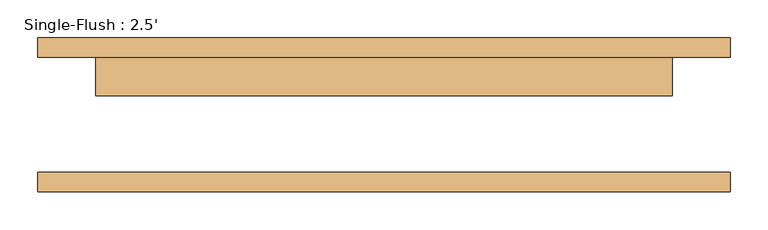
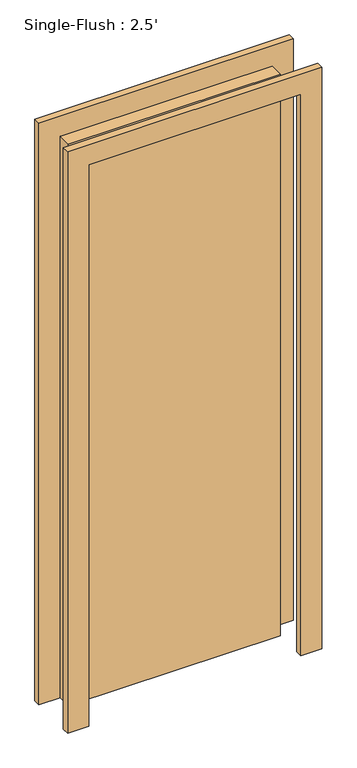
"""IFC4 building model written with IfcOpenShell, lengths in millimetres: door geometry, Single-Flush : 2.5'."""

from ifc_helpers import new_model, si_unit, frame, origin, origin_with_axes, place, context, project, spatial, polyline, outline, extrude, source, transform, mapped, element, save


def single_flush_2_5_a9addea7(model_context):
    return source(origin(), model_context, "Body", "SweptSolid", [
        extrude(outline(polyline([(2209.8, -457.2), (0.0, -457.2), (0.0, -381.0), (2133.6, -381.0), (2133.6, 381.0), (0.0, 381.0), (0.0, 457.2), (2209.8, 457.2), (2209.8, -457.2)])), frame((0.0, 76.2, 0.0), z_axis=(0.0, 1.0, 0.0), x_axis=(0.0, 0.0, 1.0)), (0.0, 0.0, 1.0), 25.4),
        extrude(outline(polyline([(2209.8, 457.2), (2209.8, -457.2), (0.0, -457.2), (0.0, -381.0), (2133.6, -381.0), (2133.6, 381.0), (0.0, 381.0), (0.0, 457.2), (2209.8, 457.2)])), frame((0.0, -101.6, 0.0), z_axis=(0.0, 1.0, 0.0), x_axis=(0.0, 0.0, 1.0)), (0.0, 0.0, 1.0), 25.4),
        extrude(outline(polyline([(381.0, 25.4), (-381.0, 25.4), (-381.0, 76.2), (381.0, 76.2), (381.0, 25.4)])), origin_with_axes(), (0.0, 0.0, 1.0), 2133.6),
    ])


if __name__ == "__main__":
    model = new_model("IFC4")
    model_context = context("Model", 3, world=origin())
    ifc_project = project(units=[si_unit("LENGTHUNIT", "METRE", prefix="MILLI")], contexts=[model_context])
    site = spatial("IfcSite", under=ifc_project)
    building = spatial("IfcBuilding", under=site)
    placement = place(None, origin())
    single_flush_2_5_shape = single_flush_2_5_a9addea7(model_context)
    element("IfcDoor", 1, ObjectType="Single-Flush : 2.5'", at=placement, inside=building, context=model_context, shape_type="MappedRepresentation", body=[
        mapped(single_flush_2_5_shape, transform((0.0, 0.0, 0.0), x_axis=(1.0, 0.0, 0.0), y_axis=(0.0, 1.0, 0.0), z_axis=(0.0, 0.0, 1.0))),
    ])
    save(model, "model.ifc")

# Revit data of these elements
# Type "Single-Flush : 2.5'"
#   Type Mark = "9"
#   Construction Type Id = "MDOOR"
#   Assembly Code = "C1020"
#   Analytic Construction = "Metal"
#   Thickness = 0' - 2"
#   Heat Transfer Coefficient (U) = 0.651978 BTU/(h·ft²·°F)
#   Height = 7' - 0"
#   Trim Projection Ext = 0' - 1"
#   Trim Projection Int = 0' - 1"
#   Trim Width = 0' - 3"
#   Width = 2' - 6"
#   Define Thermal Properties by = 1
#   Door Material = Door - Panel
#   Frame Material = Door - Frame
#   Visual Light Transmittance = 0
#   Solar Heat Gain Coefficient = 0
#   Function = (empty or 0)
#   Wall Closure = (empty or 0)
# Element 1 (IfcDoor, "Single-Flush : 2.5'")
#   Materials on its faces: "Door - Frame", "Door - Panel"
# Materials
#   "Door - Panel": class "Wood", colour RGB 210 159 95, transparency 0
#   "Door - Frame": colour RGB 118 70 51, transparency 0
